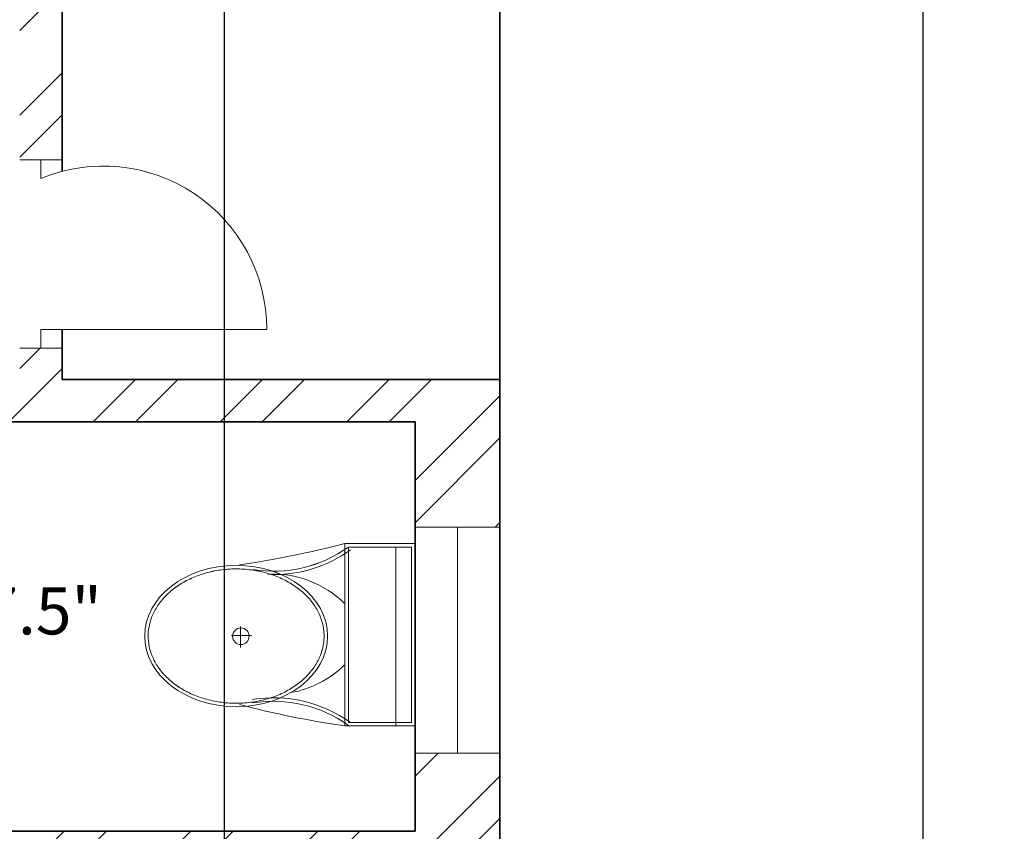
# Model space of a CAD drawing. Units: inches. Extents: x 2120 to 4013, y 1390 to 3019.
# Tile 25 of 59: x 2959 to 3063, y 1792 to 1878. Entities that reach past the tile are written whole.
import ezdxf

# ---------------------------------------------------------------- set-up
doc = ezdxf.new("R2010")
doc.units = ezdxf.units.IN
for name, color, linetype, lineweight in [('A-ANNO-DIMS', 2, 'Continuous', 18), ('A-AREA-IDEN', 7, 'Continuous', 18), ('A-DOOR', 3, 'Continuous', 18), ('A-FLOR-FIXT', 9, 'Continuous', 18), ('A-GLAZ', 4, 'Continuous', 18), ('A-WALL', 7, 'Continuous', 35), ('A-WALL-PATT', 252, 'Continuous', 13)]:
    doc.layers.add(name, color=color, linetype=linetype, lineweight=lineweight)
doc.styles.get("Standard").update_dxf_attribs({"font": 'arial.ttf'})
doc.dimstyles.get("Standard").update_dxf_attribs({"dimtxt": 0.18, "dimasz": 0.18, "dimexe": 0.18, "dimexo": 0.0625, "dimgap": 0.09, "dimtad": 0, "dimtih": 1, "dimtoh": 1, "dimdec": 4, "dimzin": 0, "dimdsep": 46, "dimtxsty": 'Standard', "dimcen": 0.09, "dimadec": 0, "dimazin": 0, "dimtfac": 1, "dimtdec": 4, "dimtofl": 0, "dimtmove": 0, "dimatfit": 3, "dimfxl": 1, "dimtolj": 1, "dimtzin": 0, "dimarcsym": 0})

# ---------------------------------------------------------------- blocks, each defined once
blk = doc.blocks.new('A$C31115884')
for p, q in [((257.5, 466.4), (257.5, 523.2)), ((283.1, 497.7), (223.4, 497.7)), ((0, 200), (0, 0)), ((520, 200), (0, 200)), ((520, 0), (520, 200)), ((10, 190), (10, 10)), ((510, 190), (10, 190)), ((510, 10), (510, 190)), ((510, 54.5), (0, 54.5)), ((10, 10), (510, 10)), ((0, 0), (520, 0))]:
    blk.add_line(p, q)
blk.add_circle((255.6, 496.4), 23.6)
for centre, radius, start, end in [((2777.7, -204.6), 2807, 165.4549, 171.7133), ((3237, 905), 2807, 188.2867, 194.5451), ((-294.5, 403.3), 364.7, 324.2091, 9.3499), ((-294.5, 403.3), 374.7, 324.2091, 9.3499), ((805.8, 403.3), 364.7, 170.6501, 215.7909), ((139.5, 406.2), 293.5, 315.8436, 2.6563), ((805.8, 403.3), 374.7, 179.2036, 215.7909), ((383.6, 406.2), 293.5, 190.2774, 224.1564)]:
    blk.add_arc(centre, radius, start, end)
blk.add_ellipse((256.2, 509.9), major_axis=(0, -260.7), ratio=0.772727)
blk.add_open_spline([(256.2, 259.2), (263.1, 259.2), (270, 259.7), (287.8, 262.3), (298.7, 265.1), (319.9, 273.1), (330.2, 278.4), (350.1, 291.1), (359.7, 298.7), (377.7, 315.9), (386.2, 325.5), (401.7, 346.6), (408.8, 358.1), (421.3, 382.5), (426.8, 395.5), (435.9, 422.4), (439.5, 436.4), (444.8, 465.1), (446.5, 479.7), (447.9, 509.2), (447.6, 524), (445, 553.3), (442.7, 567.8), (436.3, 596), (432.1, 609.7), (421.9, 636), (416, 648.6), (402.5, 672.1), (395, 683), (378.6, 703), (369.8, 712.1), (351.1, 728), (341.3, 734.8), (320.9, 746.2), (310.4, 750.7), (288.9, 757.3), (278, 759.4), (256, 761), (245, 760.6), (223.1, 757.2), (212.3, 754.3), (191.1, 746.1), (180.8, 740.7), (160.9, 727.8), (151.4, 720.1), (133.5, 702.7), (125.1, 693), (109.6, 671.7), (102.6, 660.2), (90.2, 635.7), (84.9, 622.7), (76, 595.6), (72.4, 581.6), (67.2, 552.9), (65.6, 538.2), (64.4, 508.8), (64.8, 494), (67.5, 464.7), (69.9, 450.2), (76.6, 422), (80.8, 408.3), (91.1, 382.2), (97.2, 369.7), (110.8, 346.3), (118.4, 335.4), (134.8, 315.6), (143.7, 306.7), (162.4, 290.9), (172.3, 284.2), (192.8, 273), (203.3, 268.6), (224.8, 262.2), (235.8, 260.2), (249.9, 259.3), (253, 259.2), (256.2, 259.2)], degree=3, knots=[0, 0, 0, 0, 0.110105, 0.110105, 0.285049, 0.285049, 0.459994, 0.459994, 0.634938, 0.634938, 0.809882, 0.809882, 0.984827, 0.984827, 1.159771, 1.159771, 1.334715, 1.334715, 1.50966, 1.50966, 1.684604, 1.684604, 1.859549, 1.859549, 2.034493, 2.034493, 2.209437, 2.209437, 2.384382, 2.384382, 2.559326, 2.559326, 2.73427, 2.73427, 2.909215, 2.909215, 3.084159, 3.084159, 3.259103, 3.259103, 3.434048, 3.434048, 3.608992, 3.608992, 3.783936, 3.783936, 3.958881, 3.958881, 4.133825, 4.133825, 4.30877, 4.30877, 4.483714, 4.483714, 4.658658, 4.658658, 4.833603, 4.833603, 5.008547, 5.008547, 5.183491, 5.183491, 5.358436, 5.358436, 5.53338, 5.53338, 5.708324, 5.708324, 5.883269, 5.883269, 6.058213, 6.058213, 6.233158, 6.233158, 6.283185, 6.283185, 6.283185, 6.283185])
blk = doc.blocks.new('DOOR-SWING-24IN-112p55DEG')
for p, q in [((0, 20.02), (4.5, 20.02)), ((4.5, 20.02), (2.25, 20.02)), ((2.25, 20.02), (2.25, 18.02)), ((2.25, 0), (2.25, 2)), ((2.25, 2), (26.25, 2)), ((0, 0), (4.5, 0)), ((4.5, 0), (2.25, 0))]:
    blk.add_line(p, q)
blk.add_arc((8.9, 2), 17.35, 0, 112.5501)
blk = doc.blocks.new('WIN-PLAN-24IN-05')
for p, q in [((4.5, 24), (0, 24)), ((0, 24), (9, 24)), ((4.5, 0), (4.5, 24)), ((0, 0), (9, 0)), ((9, 0), (0, 0)), ((0, 0), (4.5, 0))]:
    blk.add_line(p, q)
blk = doc.blocks.new('*D212')
at = {"layer": 'A-ANNO-DIMS', "color": 0, "lineweight": -2, "transparency": 16777216}
for p, q in [((3009.8, 2352.53), (3054.91, 2352.53)), ((3054.73, 2352.35), (3054.73, 1947.71)), ((3054.73, 1542.71), (3054.73, 1947.35)), ((3009.8, 1542.53), (3054.91, 1542.53))]:
    blk.add_line(p, q, dxfattribs=at)
at = {"layer": 'A-ANNO-DIMS', "color": 0, "transparency": 16777216}
for points in [[(3054.7, 2352.35), (3054.76, 2352.35), (3054.73, 2352.53)], [(3054.7, 1542.71), (3054.76, 1542.71), (3054.73, 1542.53)]]:
    blk.add_solid(points, dxfattribs=at)
at = {"layer": 'Defpoints', "color": 0, "transparency": 16777216}
for p in [(3009.73, 2352.53), (3009.73, 1542.53), (3054.73, 1542.53)]:
    blk.add_point(p, dxfattribs=at)
at = {"layer": 'A-ANNO-DIMS', "color": 0, "transparency": 16777216, "insert": (3054.73, 1947.53), "char_height": 0.18, "attachment_point": 5}
blk.add_mtext('\\A1;810', dxfattribs=at)
blk = doc.blocks.new('*D217')
at = {"layer": 'A-ANNO-DIMS', "color": 0, "lineweight": -2, "transparency": 16777216}
for p, q in [((3071.67, 2352.53), (2980.31, 2352.53)), ((2980.49, 2352.35), (2980.49, 1947.71)), ((2980.49, 1542.71), (2980.49, 1947.35)), ((3305.67, 1542.53), (2980.31, 1542.53))]:
    blk.add_line(p, q, dxfattribs=at)
at = {"layer": 'A-ANNO-DIMS', "color": 0, "transparency": 16777216}
for points in [[(2980.46, 2352.35), (2980.52, 2352.35), (2980.49, 2352.53)], [(2980.46, 1542.71), (2980.52, 1542.71), (2980.49, 1542.53)]]:
    blk.add_solid(points, dxfattribs=at)
at = {"layer": 'Defpoints', "color": 0, "transparency": 16777216}
for p in [(2980.49, 2352.53), (3071.73, 2352.53), (3305.73, 1542.53)]:
    blk.add_point(p, dxfattribs=at)
at = {"layer": 'A-ANNO-DIMS', "color": 0, "transparency": 16777216, "insert": (2980.49, 1947.53), "char_height": 0.18, "attachment_point": 5}
blk.add_mtext('\\A1;810', dxfattribs=at)

msp = doc.modelspace()

# ---------------------------------------------------------------- hatches: boundary and pattern name
at = {"layer": 'A-WALL-PATT'}
h = msp.add_hatch(dxfattribs=at)
h.set_pattern_fill('ANSI32', color=256)
h.paths.add_polyline_path([(2271.7331, 2343.531), (2283.3788, 2343.531), (2283.3788, 2348.031), (2283.3788, 2352.5306), (2262.7331, 2352.5306), (2262.7331, 2182.638), (2267.2331, 2182.638), (2271.7331, 2182.638), (2271.7331, 2219.031), (2391.7331, 2219.031), (2391.7331, 2214.189), (2393.9831, 2214.189), (2396.2331, 2214.189), (2396.2331, 2219.031), (2420.2331, 2219.031), (2420.2331, 2225.7535), (2417.2197, 2225.7535), (2415.7331, 2225.7535), (2415.7331, 2223.5306), (2271.7331, 2223.5306)])
h.paths.add_polyline_path([(2380.0942, 2352.5306), (2343.3788, 2352.5306), (2343.3788, 2343.531), (2363.2331, 2343.531), (2363.2331, 2288.8489), (2365.4831, 2288.8489), (2367.7331, 2288.8489), (2367.7331, 2343.531), (2380.0942, 2343.531)], flags=17)
h.paths.add_polyline_path([(2432.4339, 2352.5306), (2404.0943, 2352.5306), (2404.0943, 2343.531), (2415.7331, 2343.531), (2415.7331, 2264.0306), (2367.7331, 2264.0306), (2367.7331, 2266.4872), (2363.2331, 2266.4872), (2363.2331, 2259.531), (2367.7331, 2259.531), (2415.7331, 2259.531), (2415.7331, 2255.0658), (2420.2331, 2255.0658), (2420.2331, 2259.531), (2424.5717, 2259.531), (2424.5717, 2261.781), (2424.5717, 2264.0306), (2420.2331, 2264.0306), (2420.2331, 2343.531), (2432.4339, 2343.531)])
h.paths.add_polyline_path([(2508.9115, 2352.5306), (2456.4339, 2352.5306), (2456.4339, 2343.531), (2468.2331, 2343.531), (2468.2331, 2264.0306), (2448.0487, 2264.0306), (2448.0487, 2259.531), (2468.2331, 2259.531), (2468.2331, 2255.5496), (2472.7331, 2255.5496), (2472.7331, 2343.531), (2508.9115, 2343.531)])
h.paths.add_polyline_path([(2637.7331, 2352.5306), (2544.9116, 2352.5306), (2544.9116, 2343.531), (2589.7331, 2343.531), (2633.2331, 2343.531), (2637.7331, 2343.531)])
h.paths.add_polyline_path([(2594.2331, 2343.5306), (2589.7331, 2343.5306), (2589.7331, 2259.5306), (2589.7331, 2252.4915), (2591.9831, 2252.4915), (2594.2331, 2252.4915)])
h.paths.add_polyline_path([(2637.7331, 2223.5306), (2594.2331, 2223.5306), (2594.2331, 2230.1988), (2591.9831, 2230.1988), (2589.7331, 2230.1988), (2589.7331, 2223.5306), (2472.7331, 2223.5306), (2468.2331, 2223.5306), (2468.2331, 2219.031), (2628.7331, 2219.031), (2628.7331, 2138.031), (2637.7331, 2138.031)])
h.paths.add_polyline_path([(3822.6535, 2458.4402), (3874.9468, 2458.4402), (3874.9468, 2476.9866), (3822.6535, 2476.9866)], flags=9)
h.paths.add_polyline_path([(3834.6921, 2781.8174), (3935.9206, 2781.8174), (3935.9206, 2800.3638), (3834.6921, 2800.3638)], flags=9)
h.paths.add_polyline_path([(3832.2843, 2837.9683), (3884.5776, 2837.9683), (3884.5776, 2856.5146), (3832.2843, 2856.5146)], flags=9)
h.paths.add_polyline_path([(3830.9388, 2861.4782), (3956.8958, 2861.4782), (3956.8958, 2880.0245), (3830.9388, 2880.0245)], flags=9)
h.paths.add_polyline_path([(3870.6966, 2352.5752), (3887.9272, 2352.5752), (3887.9272, 2377.3037), (3870.6966, 2377.3037)], flags=9)
h.paths.add_polyline_path([(3289.2701, 2413.161), (3435.2223, 2413.161), (3435.2223, 2450.2538), (3289.2701, 2450.2538)], flags=9)
h.paths.add_polyline_path([(2487.6944, 2414.3601), (2637.8335, 2414.3601), (2637.8335, 2451.4528), (2487.6944, 2451.4528)], flags=9)
h.paths.add_polyline_path([(2567.3724, 1457.9199), (2815.296, 1457.9199), (2815.296, 1495.0127), (2567.3724, 1495.0127)], flags=9)
h.paths.add_polyline_path([(2655.3825, 2093.2363), (2685.9555, 2093.2363), (2685.9555, 2111.8937), (2655.3825, 2111.8937)], flags=9)
h.paths.add_polyline_path([(2543.9218, 1550.6671), (2587.8406, 1550.6671), (2587.8406, 1569.3244), (2543.9218, 1569.3244)], flags=9)
h.paths.add_polyline_path([(2905.1384, 1543.8113), (2949.0572, 1543.8113), (2949.0572, 1562.4686), (2905.1384, 1562.4686)], flags=9)
h.paths.add_polyline_path([(2736.4118, 1702.4736), (2784.2153, 1702.4736), (2784.2153, 1721.1309), (2736.4118, 1721.1309)], flags=9)
h.paths.add_polyline_path([(2912.8666, 1710.4168), (2951.707, 1710.4168), (2951.707, 1729.0741), (2912.8666, 1729.0741)], flags=9)
h.paths.add_polyline_path([(2923.5785, 1763.5038), (2959.7279, 1763.5038), (2959.7279, 1782.1611), (2923.5785, 1782.1611)], flags=9)
h.paths.add_polyline_path([(2925.2114, 1809.6137), (2967.1861, 1809.6137), (2967.1861, 1828.271), (2925.2114, 1828.271)], flags=9)
h.paths.add_polyline_path([(2996.2711, 1878.9003), (2996.2711, 1913.109), (2977.6138, 1913.109), (2977.6138, 1878.9003)], flags=9)
h.paths.add_polyline_path([(2883.0859, 1895.7192), (2927.1855, 1895.7192), (2927.1855, 1914.3766), (2883.0859, 1914.3766)], flags=9)
h.paths.add_polyline_path([(2787.3924, 1810.8013), (2841.0213, 1810.8013), (2841.0213, 1829.4587), (2787.3924, 1829.4587)], flags=9)
h.paths.add_polyline_path([(2775.6399, 2101.7395), (2829.2689, 2101.7395), (2829.2689, 2120.3968), (2775.6399, 2120.3968)], flags=9)
h.paths.add_polyline_path([(2913.0263, 2075.817), (2951.8667, 2075.817), (2951.8667, 2094.4744), (2913.0263, 2094.4744)], flags=9)
h.paths.add_polyline_path([(2929.966, 2133.3669), (2966.1154, 2133.3669), (2966.1154, 2152.0243), (2929.966, 2152.0243)], flags=9)
h.paths.add_polyline_path([(2932.7502, 2182.6088), (2968.8996, 2182.6088), (2968.8996, 2201.2662), (2932.7502, 2201.2662)], flags=9)
h.paths.add_polyline_path([(2996.0681, 2266.3173), (2996.0681, 2300.5261), (2977.4108, 2300.5261), (2977.4108, 2266.3173)], flags=9)
h.paths.add_polyline_path([(2885.1039, 2279.2186), (2929.2035, 2279.2186), (2929.2035, 2297.8759), (2885.1039, 2297.8759)], flags=9)
h.paths.add_polyline_path([(2735.7042, 2218.3197), (2783.5078, 2218.3197), (2783.5078, 2236.9771), (2735.7042, 2236.9771)], flags=9)
h.paths.add_polyline_path([(2635.6049, 2044.0085), (2648.9678, 2044.0085), (2648.9678, 2054.312), (2635.6049, 2054.312)], flags=9)
h.paths.add_polyline_path([(2714.0148, 1923.0473), (2727.3777, 1923.0473), (2727.3777, 1933.3508), (2714.0148, 1933.3508)], flags=9)
h.paths.add_polyline_path([(2709.0345, 1988.1628), (2722.3974, 1988.1628), (2722.3974, 1998.4663), (2709.0345, 1998.4663)], flags=9)
h.paths.add_polyline_path([(2592.8935, 1962.1763), (2606.2564, 1962.1763), (2606.2564, 1972.4799), (2592.8935, 1972.4799)], flags=9)
h.paths.add_polyline_path([(2618.3996, 1985.9724), (2644.1942, 1985.9724), (2644.1942, 1996.2759), (2618.3996, 1996.2759)], flags=9)
h.paths.add_polyline_path([(2601.279, 1920.5869), (2614.6419, 1920.5869), (2614.6419, 1930.8904), (2601.279, 1930.8904)], flags=9)
h.paths.add_polyline_path([(2692.3278, 1932.7645), (2704.5311, 1932.7645), (2704.5311, 1943.0681), (2692.3278, 1943.0681)], flags=9)
h.paths.add_polyline_path([(2311.122, 1672.7318), (2355.0408, 1672.7318), (2355.0408, 1691.3892), (2311.122, 1691.3892)], flags=9)
h.paths.add_polyline_path([(2456.2551, 1632.3198), (2492.4796, 1632.3198), (2492.4796, 1650.9772), (2456.2551, 1650.9772)], flags=9)
h.paths.add_polyline_path([(2401.0766, 1631.4793), (2437.301, 1631.4793), (2437.301, 1650.1367), (2401.0766, 1650.1367)], flags=9)
h.paths.add_polyline_path([(2546.7054, 1700.9235), (2594.509, 1700.9235), (2594.509, 1719.5809), (2546.7054, 1719.5809)], flags=9)
h.paths.add_polyline_path([(2445.4866, 1766.9937), (2497.5261, 1766.9937), (2497.5261, 1785.651), (2445.4866, 1785.651)], flags=9)
h.paths.add_polyline_path([(2287.9992, 1739.7675), (2326.8396, 1739.7675), (2326.8396, 1758.4248), (2287.9992, 1758.4248)], flags=9)
h.paths.add_polyline_path([(2458.5279, 1924.7607), (2510.5675, 1924.7607), (2510.5675, 1943.4181), (2458.5279, 1943.4181)], flags=9)
h.paths.add_polyline_path([(2309.2811, 1902.7642), (2345.4305, 1902.7642), (2345.4305, 1921.4215), (2309.2811, 1921.4215)], flags=9)
h.paths.add_polyline_path([(2490.7554, 2018.9392), (2530.7896, 2018.9392), (2530.7896, 2037.5965), (2490.7554, 2037.5965)], flags=9)
h.paths.add_polyline_path([(2402.143, 2024.7393), (2438.5414, 2024.7393), (2438.5414, 2043.3966), (2402.143, 2043.3966)], flags=9)
h.paths.add_polyline_path([(2287.856, 1931.7926), (2326.6964, 1931.7926), (2326.6964, 1950.4499), (2287.856, 1950.4499)], flags=9)
h.paths.add_polyline_path([(2281.7979, 2193.5771), (2320.6383, 2193.5771), (2320.6383, 2212.2344), (2281.7979, 2212.2344)], flags=25)
h.paths.add_polyline_path([(2484.0754, 2093.892), (2536.115, 2093.892), (2536.115, 2112.5494), (2484.0754, 2112.5494)], flags=9)
h.paths.add_polyline_path([(2624.7948, 2281.8639), (2624.7948, 2311.4137), (2606.1375, 2311.4137), (2606.1375, 2281.8639)], flags=9)
h.paths.add_polyline_path([(2507.5036, 2290.3639), (2541.934, 2290.3639), (2541.934, 2309.0212), (2507.5036, 2309.0212)], flags=9)
h.paths.add_polyline_path([(2423.1076, 2285.2202), (2459.332, 2285.2202), (2459.332, 2303.8776), (2423.1076, 2303.8776)], flags=9)
h.paths.add_polyline_path([(2374.5467, 2289.6272), (2410.7711, 2289.6272), (2410.7711, 2308.2846), (2374.5467, 2308.2846)], flags=25)
h.paths.add_polyline_path([(2277.4907, 2227.5651), (2316.3311, 2227.5651), (2316.3311, 2246.2224), (2277.4907, 2246.2224)], flags=25)
h.paths.add_polyline_path([(2655.3825, 2093.2367), (2685.9555, 2093.2367), (2685.9555, 2111.894), (2655.3825, 2111.894)], flags=9)
h.paths.add_polyline_path([(2543.9217, 1550.6674), (2587.8406, 1550.6674), (2587.8406, 1569.3247), (2543.9217, 1569.3247)], flags=9)
h.paths.add_polyline_path([(2905.1384, 1543.8116), (2949.0572, 1543.8116), (2949.0572, 1562.4689), (2905.1384, 1562.4689)], flags=9)
h.paths.add_polyline_path([(2736.4118, 1702.4739), (2784.2153, 1702.4739), (2784.2153, 1721.1312), (2736.4118, 1721.1312)], flags=9)
h.paths.add_polyline_path([(2912.8666, 1710.4171), (2951.707, 1710.4171), (2951.707, 1729.0744), (2912.8666, 1729.0744)], flags=9)
h.paths.add_polyline_path([(2923.5785, 1763.5041), (2959.7279, 1763.5041), (2959.7279, 1782.1614), (2923.5785, 1782.1614)], flags=9)
h.paths.add_polyline_path([(2925.2114, 1809.614), (2967.1861, 1809.614), (2967.1861, 1828.2713), (2925.2114, 1828.2713)], flags=9)
h.paths.add_polyline_path([(2996.2711, 1878.9006), (2996.2711, 1913.1094), (2977.6137, 1913.1094), (2977.6137, 1878.9006)], flags=9)
h.paths.add_polyline_path([(2883.0859, 1895.7195), (2927.1855, 1895.7195), (2927.1855, 1914.3769), (2883.0859, 1914.3769)], flags=9)
h.paths.add_polyline_path([(2787.3924, 1810.8016), (2841.0213, 1810.8016), (2841.0213, 1829.459), (2787.3924, 1829.459)], flags=9)
h.paths.add_polyline_path([(2775.6399, 2101.7398), (2829.2688, 2101.7398), (2829.2688, 2120.3971), (2775.6399, 2120.3971)], flags=9)
h.paths.add_polyline_path([(2913.0263, 2075.8173), (2951.8667, 2075.8173), (2951.8667, 2094.4747), (2913.0263, 2094.4747)], flags=9)
h.paths.add_polyline_path([(2929.966, 2133.3672), (2966.1154, 2133.3672), (2966.1154, 2152.0246), (2929.966, 2152.0246)], flags=9)
h.paths.add_polyline_path([(2932.7502, 2182.6091), (2968.8996, 2182.6091), (2968.8996, 2201.2665), (2932.7502, 2201.2665)], flags=9)
h.paths.add_polyline_path([(2996.0681, 2266.3176), (2996.0681, 2300.5264), (2977.4108, 2300.5264), (2977.4108, 2266.3176)], flags=9)
h.paths.add_polyline_path([(2885.1039, 2279.2189), (2929.2035, 2279.2189), (2929.2035, 2297.8762), (2885.1039, 2297.8762)], flags=9)
h.paths.add_polyline_path([(2735.7042, 2218.32), (2783.5078, 2218.32), (2783.5078, 2236.9774), (2735.7042, 2236.9774)], flags=9)
h.paths.add_polyline_path([(2635.6048, 2044.0088), (2648.9677, 2044.0088), (2648.9677, 2054.3123), (2635.6048, 2054.3123)], flags=9)
h.paths.add_polyline_path([(2714.0148, 1923.0476), (2727.3777, 1923.0476), (2727.3777, 1933.3511), (2714.0148, 1933.3511)], flags=9)
h.paths.add_polyline_path([(2709.0345, 1988.1631), (2722.3974, 1988.1631), (2722.3974, 1998.4666), (2709.0345, 1998.4666)], flags=9)
h.paths.add_polyline_path([(2592.8935, 1962.1766), (2606.2564, 1962.1766), (2606.2564, 1972.4802), (2592.8935, 1972.4802)], flags=9)
h.paths.add_polyline_path([(2618.3995, 1985.9727), (2644.1942, 1985.9727), (2644.1942, 1996.2762), (2618.3995, 1996.2762)], flags=9)
h.paths.add_polyline_path([(2601.279, 1920.5872), (2614.6419, 1920.5872), (2614.6419, 1930.8908), (2601.279, 1930.8908)], flags=9)
h.paths.add_polyline_path([(2692.3278, 1932.7648), (2704.5311, 1932.7648), (2704.5311, 1943.0684), (2692.3278, 1943.0684)], flags=9)
h.paths.add_polyline_path([(2311.122, 1672.7321), (2355.0408, 1672.7321), (2355.0408, 1691.3895), (2311.122, 1691.3895)], flags=9)
h.paths.add_polyline_path([(2456.2551, 1632.3201), (2492.4795, 1632.3201), (2492.4795, 1650.9775), (2456.2551, 1650.9775)], flags=9)
h.paths.add_polyline_path([(2401.0766, 1631.4796), (2437.301, 1631.4796), (2437.301, 1650.137), (2401.0766, 1650.137)], flags=9)
h.paths.add_polyline_path([(2546.7054, 1700.9238), (2594.509, 1700.9238), (2594.509, 1719.5812), (2546.7054, 1719.5812)], flags=9)
h.paths.add_polyline_path([(2445.4866, 1766.994), (2497.5261, 1766.994), (2497.5261, 1785.6513), (2445.4866, 1785.6513)], flags=9)
h.paths.add_polyline_path([(2287.9992, 1739.7678), (2326.8396, 1739.7678), (2326.8396, 1758.4251), (2287.9992, 1758.4251)], flags=9)
h.paths.add_polyline_path([(2458.5279, 1924.7611), (2510.5675, 1924.7611), (2510.5675, 1943.4184), (2458.5279, 1943.4184)], flags=9)
h.paths.add_polyline_path([(2309.2811, 1902.7645), (2345.4305, 1902.7645), (2345.4305, 1921.4218), (2309.2811, 1921.4218)], flags=9)
h.paths.add_polyline_path([(2490.7554, 2018.9395), (2530.7895, 2018.9395), (2530.7895, 2037.5968), (2490.7554, 2037.5968)], flags=9)
h.paths.add_polyline_path([(2402.143, 2024.7396), (2438.5413, 2024.7396), (2438.5413, 2043.3969), (2402.143, 2043.3969)], flags=9)
h.paths.add_polyline_path([(2287.856, 1931.7929), (2326.6964, 1931.7929), (2326.6964, 1950.4502), (2287.856, 1950.4502)], flags=9)
h.paths.add_polyline_path([(2281.7979, 2193.5774), (2320.6383, 2193.5774), (2320.6383, 2212.2347), (2281.7979, 2212.2347)], flags=25)
h.paths.add_polyline_path([(2484.0754, 2093.8924), (2536.115, 2093.8924), (2536.115, 2112.5497), (2484.0754, 2112.5497)], flags=9)
h.paths.add_polyline_path([(2624.7948, 2281.8642), (2624.7948, 2311.414), (2606.1374, 2311.414), (2606.1374, 2281.8642)], flags=9)
h.paths.add_polyline_path([(2507.5035, 2290.3642), (2541.934, 2290.3642), (2541.934, 2309.0215), (2507.5035, 2309.0215)], flags=9)
h.paths.add_polyline_path([(2423.1075, 2285.2205), (2459.332, 2285.2205), (2459.332, 2303.8779), (2423.1075, 2303.8779)], flags=9)
h.paths.add_polyline_path([(2374.5467, 2289.6275), (2410.7711, 2289.6275), (2410.7711, 2308.2849), (2374.5467, 2308.2849)], flags=25)
h.paths.add_polyline_path([(2277.4907, 2227.5654), (2316.3311, 2227.5654), (2316.3311, 2246.2227), (2277.4907, 2246.2227)], flags=25)
h = msp.add_hatch(dxfattribs=at)
h.set_pattern_fill('ANSI32', color=256)
h.paths.add_polyline_path([(2271.7331, 1980.389), (2262.7331, 1980.389), (2262.7331, 1912.8434), (2267.2331, 1912.8434), (2271.7331, 1912.8434), (2271.7331, 1922.531), (2351.2331, 1922.531), (2351.2331, 1901.4728), (2355.7331, 1901.4728), (2355.7331, 1922.531), (2357.9815, 1922.531), (2357.9815, 1926.5306), (2271.7331, 1926.5306)])
h.paths.add_polyline_path([(2589.2331, 1949.1622), (2584.7331, 1949.1622), (2580.2331, 1949.1622), (2580.2331, 1874.5306), (2355.7331, 1874.5306), (2355.7331, 1880.1922), (2351.2331, 1880.1922), (2351.2331, 1874.5306), (2271.7331, 1874.5306), (2271.7331, 1888.8431), (2262.7331, 1888.8431), (2262.7331, 1842.2909), (2267.2331, 1842.2909), (2271.7331, 1842.2909), (2271.7331, 1865.531), (2415.7331, 1865.531), (2415.7331, 1779.7286), (2420.2331, 1779.7286), (2420.2331, 1865.531), (2589.2331, 1865.531)])
h.paths.add_polyline_path([(2271.7331, 1782.2906), (2262.7331, 1782.2906), (2262.7331, 1711.4639), (2267.2331, 1711.4639), (2271.7331, 1711.4639), (2271.7331, 1738.031), (2420.2331, 1738.031), (2420.2331, 1742.531), (2420.2331, 1747.3376), (2417.9831, 1747.3376), (2415.7331, 1747.3376), (2415.7331, 1742.5306), (2271.7331, 1742.5306)])
h.paths.add_polyline_path([(2271.7331, 1627.031), (2362.3957, 1627.031), (2362.3957, 1629.281), (2362.3957, 1631.5306), (2271.7331, 1631.5306), (2271.7331, 1675.4636), (2262.7331, 1675.4636), (2262.7331, 1581.531), (2405.3032, 1581.531), (2405.3032, 1586.031), (2405.3032, 1590.5306), (2396.2331, 1590.5306), (2396.2331, 1691.4513), (2418.7206, 1691.4513), (2418.7206, 1695.951), (2396.2331, 1695.951), (2391.7331, 1695.951), (2391.7331, 1631.5306), (2386.7425, 1631.5306), (2386.7425, 1629.2806), (2386.7425, 1627.031), (2391.7331, 1627.031), (2391.7331, 1586.1709), (2271.7331, 1586.1709)])
h.paths.add_polyline_path([(2459.6703, 1590.5306), (2429.3032, 1590.5306), (2429.3032, 1581.531), (2459.6703, 1581.531), (2459.6703, 1586.031)])
h.paths.add_polyline_path([(2501.2331, 1590.531), (2501.2331, 1665.0195), (2498.9831, 1665.0195), (2496.7331, 1665.0195), (2496.7331, 1590.5306), (2483.8201, 1590.5306), (2483.8201, 1590.1579), (2483.6704, 1590.1579), (2483.6704, 1581.531), (2505.0196, 1581.531), (2505.0196, 1583.781), (2505.0196, 1586.0306), (2501.2331, 1586.0306)])
h.paths.add_polyline_path([(2544.1361, 1583.781), (2544.1361, 1586.0306), (2527.1368, 1586.0306), (2527.1368, 1583.7806), (2527.1368, 1581.531), (2544.1361, 1581.531)])
h.paths.add_polyline_path([(3822.6535, 2458.4402), (3874.9468, 2458.4402), (3874.9468, 2476.9866), (3822.6535, 2476.9866)], flags=9)
h.paths.add_polyline_path([(3834.6921, 2781.8174), (3935.9206, 2781.8174), (3935.9206, 2800.3638), (3834.6921, 2800.3638)], flags=9)
h.paths.add_polyline_path([(3832.2843, 2837.9683), (3884.5776, 2837.9683), (3884.5776, 2856.5146), (3832.2843, 2856.5146)], flags=9)
h.paths.add_polyline_path([(3830.9388, 2861.4782), (3956.8958, 2861.4782), (3956.8958, 2880.0245), (3830.9388, 2880.0245)], flags=9)
h.paths.add_polyline_path([(3870.6966, 2352.5752), (3887.9272, 2352.5752), (3887.9272, 2377.3037), (3870.6966, 2377.3037)], flags=9)
h.paths.add_polyline_path([(3289.2701, 2413.161), (3435.2223, 2413.161), (3435.2223, 2450.2538), (3289.2701, 2450.2538)], flags=9)
h.paths.add_polyline_path([(2487.6944, 2414.3601), (2637.8335, 2414.3601), (2637.8335, 2451.4528), (2487.6944, 2451.4528)], flags=9)
h.paths.add_polyline_path([(2567.3724, 1457.9199), (2815.296, 1457.9199), (2815.296, 1495.0127), (2567.3724, 1495.0127)], flags=9)
h.paths.add_polyline_path([(2655.3825, 2093.2363), (2685.9555, 2093.2363), (2685.9555, 2111.8937), (2655.3825, 2111.8937)], flags=9)
h.paths.add_polyline_path([(2543.9218, 1550.6671), (2587.8406, 1550.6671), (2587.8406, 1569.3244), (2543.9218, 1569.3244)], flags=9)
h.paths.add_polyline_path([(2905.1384, 1543.8113), (2949.0572, 1543.8113), (2949.0572, 1562.4686), (2905.1384, 1562.4686)], flags=9)
h.paths.add_polyline_path([(2736.4118, 1702.4736), (2784.2153, 1702.4736), (2784.2153, 1721.1309), (2736.4118, 1721.1309)], flags=9)
h.paths.add_polyline_path([(2912.8666, 1710.4168), (2951.707, 1710.4168), (2951.707, 1729.0741), (2912.8666, 1729.0741)], flags=9)
h.paths.add_polyline_path([(2923.5785, 1763.5038), (2959.7279, 1763.5038), (2959.7279, 1782.1611), (2923.5785, 1782.1611)], flags=9)
h.paths.add_polyline_path([(2925.2114, 1809.6137), (2967.1861, 1809.6137), (2967.1861, 1828.271), (2925.2114, 1828.271)], flags=9)
h.paths.add_polyline_path([(2996.2711, 1878.9003), (2996.2711, 1913.109), (2977.6138, 1913.109), (2977.6138, 1878.9003)], flags=9)
h.paths.add_polyline_path([(2883.0859, 1895.7192), (2927.1855, 1895.7192), (2927.1855, 1914.3766), (2883.0859, 1914.3766)], flags=9)
h.paths.add_polyline_path([(2787.3924, 1810.8013), (2841.0213, 1810.8013), (2841.0213, 1829.4587), (2787.3924, 1829.4587)], flags=9)
h.paths.add_polyline_path([(2775.6399, 2101.7395), (2829.2689, 2101.7395), (2829.2689, 2120.3968), (2775.6399, 2120.3968)], flags=9)
h.paths.add_polyline_path([(2913.0263, 2075.817), (2951.8667, 2075.817), (2951.8667, 2094.4744), (2913.0263, 2094.4744)], flags=9)
h.paths.add_polyline_path([(2929.966, 2133.3669), (2966.1154, 2133.3669), (2966.1154, 2152.0243), (2929.966, 2152.0243)], flags=9)
h.paths.add_polyline_path([(2932.7502, 2182.6088), (2968.8996, 2182.6088), (2968.8996, 2201.2662), (2932.7502, 2201.2662)], flags=9)
h.paths.add_polyline_path([(2996.0681, 2266.3173), (2996.0681, 2300.5261), (2977.4108, 2300.5261), (2977.4108, 2266.3173)], flags=9)
h.paths.add_polyline_path([(2885.1039, 2279.2186), (2929.2035, 2279.2186), (2929.2035, 2297.8759), (2885.1039, 2297.8759)], flags=9)
h.paths.add_polyline_path([(2735.7042, 2218.3197), (2783.5078, 2218.3197), (2783.5078, 2236.9771), (2735.7042, 2236.9771)], flags=9)
h.paths.add_polyline_path([(2635.6049, 2044.0085), (2648.9678, 2044.0085), (2648.9678, 2054.312), (2635.6049, 2054.312)], flags=9)
h.paths.add_polyline_path([(2714.0148, 1923.0473), (2727.3777, 1923.0473), (2727.3777, 1933.3508), (2714.0148, 1933.3508)], flags=9)
h.paths.add_polyline_path([(2709.0345, 1988.1628), (2722.3974, 1988.1628), (2722.3974, 1998.4663), (2709.0345, 1998.4663)], flags=9)
h.paths.add_polyline_path([(2592.8935, 1962.1763), (2606.2564, 1962.1763), (2606.2564, 1972.4799), (2592.8935, 1972.4799)], flags=9)
h.paths.add_polyline_path([(2618.3996, 1985.9724), (2644.1942, 1985.9724), (2644.1942, 1996.2759), (2618.3996, 1996.2759)], flags=9)
h.paths.add_polyline_path([(2601.279, 1920.5869), (2614.6419, 1920.5869), (2614.6419, 1930.8904), (2601.279, 1930.8904)], flags=9)
h.paths.add_polyline_path([(2692.3278, 1932.7645), (2704.5311, 1932.7645), (2704.5311, 1943.0681), (2692.3278, 1943.0681)], flags=9)
h.paths.add_polyline_path([(2311.122, 1672.7318), (2355.0408, 1672.7318), (2355.0408, 1691.3892), (2311.122, 1691.3892)], flags=25)
h.paths.add_polyline_path([(2456.2551, 1632.3198), (2492.4796, 1632.3198), (2492.4796, 1650.9772), (2456.2551, 1650.9772)], flags=9)
h.paths.add_polyline_path([(2401.0766, 1631.4793), (2437.301, 1631.4793), (2437.301, 1650.1367), (2401.0766, 1650.1367)], flags=9)
h.paths.add_polyline_path([(2546.7054, 1700.9235), (2594.509, 1700.9235), (2594.509, 1719.5809), (2546.7054, 1719.5809)], flags=9)
h.paths.add_polyline_path([(2445.4866, 1766.9937), (2497.5261, 1766.9937), (2497.5261, 1785.651), (2445.4866, 1785.651)], flags=9)
h.paths.add_polyline_path([(2287.9992, 1739.7675), (2326.8396, 1739.7675), (2326.8396, 1758.4248), (2287.9992, 1758.4248)], flags=24)
h.paths.add_polyline_path([(2458.5279, 1924.7607), (2510.5675, 1924.7607), (2510.5675, 1943.4181), (2458.5279, 1943.4181)], flags=25)
h.paths.add_polyline_path([(2309.2811, 1902.7642), (2345.4305, 1902.7642), (2345.4305, 1921.4215), (2309.2811, 1921.4215)], flags=25)
h.paths.add_polyline_path([(2490.7554, 2018.9392), (2530.7896, 2018.9392), (2530.7896, 2037.5965), (2490.7554, 2037.5965)], flags=9)
h.paths.add_polyline_path([(2402.143, 2024.7393), (2438.5414, 2024.7393), (2438.5414, 2043.3966), (2402.143, 2043.3966)], flags=9)
h.paths.add_polyline_path([(2287.856, 1931.7926), (2326.6964, 1931.7926), (2326.6964, 1950.4499), (2287.856, 1950.4499)], flags=25)
h.paths.add_polyline_path([(2281.7979, 2193.5771), (2320.6383, 2193.5771), (2320.6383, 2212.2344), (2281.7979, 2212.2344)], flags=9)
h.paths.add_polyline_path([(2484.0754, 2093.892), (2536.115, 2093.892), (2536.115, 2112.5494), (2484.0754, 2112.5494)], flags=9)
h.paths.add_polyline_path([(2624.7948, 2281.8639), (2624.7948, 2311.4137), (2606.1375, 2311.4137), (2606.1375, 2281.8639)], flags=9)
h.paths.add_polyline_path([(2507.5036, 2290.3639), (2541.934, 2290.3639), (2541.934, 2309.0212), (2507.5036, 2309.0212)], flags=9)
h.paths.add_polyline_path([(2423.1076, 2285.2202), (2459.332, 2285.2202), (2459.332, 2303.8776), (2423.1076, 2303.8776)], flags=9)
h.paths.add_polyline_path([(2374.5467, 2289.6272), (2410.7711, 2289.6272), (2410.7711, 2308.2846), (2374.5467, 2308.2846)], flags=9)
h.paths.add_polyline_path([(2277.4907, 2227.5651), (2316.3311, 2227.5651), (2316.3311, 2246.2224), (2277.4907, 2246.2224)], flags=9)
h.paths.add_polyline_path([(2655.3825, 2093.2367), (2685.9555, 2093.2367), (2685.9555, 2111.894), (2655.3825, 2111.894)], flags=9)
h.paths.add_polyline_path([(2543.9217, 1550.6674), (2587.8406, 1550.6674), (2587.8406, 1569.3247), (2543.9217, 1569.3247)], flags=9)
h.paths.add_polyline_path([(2905.1384, 1543.8116), (2949.0572, 1543.8116), (2949.0572, 1562.4689), (2905.1384, 1562.4689)], flags=9)
h.paths.add_polyline_path([(2736.4118, 1702.4739), (2784.2153, 1702.4739), (2784.2153, 1721.1312), (2736.4118, 1721.1312)], flags=9)
h.paths.add_polyline_path([(2912.8666, 1710.4171), (2951.707, 1710.4171), (2951.707, 1729.0744), (2912.8666, 1729.0744)], flags=9)
h.paths.add_polyline_path([(2923.5785, 1763.5041), (2959.7279, 1763.5041), (2959.7279, 1782.1614), (2923.5785, 1782.1614)], flags=9)
h.paths.add_polyline_path([(2925.2114, 1809.614), (2967.1861, 1809.614), (2967.1861, 1828.2713), (2925.2114, 1828.2713)], flags=9)
h.paths.add_polyline_path([(2996.2711, 1878.9006), (2996.2711, 1913.1094), (2977.6137, 1913.1094), (2977.6137, 1878.9006)], flags=9)
h.paths.add_polyline_path([(2883.0859, 1895.7195), (2927.1855, 1895.7195), (2927.1855, 1914.3769), (2883.0859, 1914.3769)], flags=9)
h.paths.add_polyline_path([(2787.3924, 1810.8016), (2841.0213, 1810.8016), (2841.0213, 1829.459), (2787.3924, 1829.459)], flags=9)
h.paths.add_polyline_path([(2775.6399, 2101.7398), (2829.2688, 2101.7398), (2829.2688, 2120.3971), (2775.6399, 2120.3971)], flags=9)
h.paths.add_polyline_path([(2913.0263, 2075.8173), (2951.8667, 2075.8173), (2951.8667, 2094.4747), (2913.0263, 2094.4747)], flags=9)
h.paths.add_polyline_path([(2929.966, 2133.3672), (2966.1154, 2133.3672), (2966.1154, 2152.0246), (2929.966, 2152.0246)], flags=9)
h.paths.add_polyline_path([(2932.7502, 2182.6091), (2968.8996, 2182.6091), (2968.8996, 2201.2665), (2932.7502, 2201.2665)], flags=9)
h.paths.add_polyline_path([(2996.0681, 2266.3176), (2996.0681, 2300.5264), (2977.4108, 2300.5264), (2977.4108, 2266.3176)], flags=9)
h.paths.add_polyline_path([(2885.1039, 2279.2189), (2929.2035, 2279.2189), (2929.2035, 2297.8762), (2885.1039, 2297.8762)], flags=9)
h.paths.add_polyline_path([(2735.7042, 2218.32), (2783.5078, 2218.32), (2783.5078, 2236.9774), (2735.7042, 2236.9774)], flags=9)
h.paths.add_polyline_path([(2635.6048, 2044.0088), (2648.9677, 2044.0088), (2648.9677, 2054.3123), (2635.6048, 2054.3123)], flags=9)
h.paths.add_polyline_path([(2714.0148, 1923.0476), (2727.3777, 1923.0476), (2727.3777, 1933.3511), (2714.0148, 1933.3511)], flags=9)
h.paths.add_polyline_path([(2709.0345, 1988.1631), (2722.3974, 1988.1631), (2722.3974, 1998.4666), (2709.0345, 1998.4666)], flags=9)
h.paths.add_polyline_path([(2592.8935, 1962.1766), (2606.2564, 1962.1766), (2606.2564, 1972.4802), (2592.8935, 1972.4802)], flags=9)
h.paths.add_polyline_path([(2618.3995, 1985.9727), (2644.1942, 1985.9727), (2644.1942, 1996.2762), (2618.3995, 1996.2762)], flags=9)
h.paths.add_polyline_path([(2601.279, 1920.5872), (2614.6419, 1920.5872), (2614.6419, 1930.8908), (2601.279, 1930.8908)], flags=9)
h.paths.add_polyline_path([(2692.3278, 1932.7648), (2704.5311, 1932.7648), (2704.5311, 1943.0684), (2692.3278, 1943.0684)], flags=9)
h.paths.add_polyline_path([(2311.122, 1672.7321), (2355.0408, 1672.7321), (2355.0408, 1691.3895), (2311.122, 1691.3895)], flags=25)
h.paths.add_polyline_path([(2456.2551, 1632.3201), (2492.4795, 1632.3201), (2492.4795, 1650.9775), (2456.2551, 1650.9775)], flags=9)
h.paths.add_polyline_path([(2401.0766, 1631.4796), (2437.301, 1631.4796), (2437.301, 1650.137), (2401.0766, 1650.137)], flags=9)
h.paths.add_polyline_path([(2546.7054, 1700.9238), (2594.509, 1700.9238), (2594.509, 1719.5812), (2546.7054, 1719.5812)], flags=9)
h.paths.add_polyline_path([(2445.4866, 1766.994), (2497.5261, 1766.994), (2497.5261, 1785.6513), (2445.4866, 1785.6513)], flags=9)
h.paths.add_polyline_path([(2287.9992, 1739.7678), (2326.8396, 1739.7678), (2326.8396, 1758.4251), (2287.9992, 1758.4251)], flags=24)
h.paths.add_polyline_path([(2458.5279, 1924.7611), (2510.5675, 1924.7611), (2510.5675, 1943.4184), (2458.5279, 1943.4184)], flags=25)
h.paths.add_polyline_path([(2309.2811, 1902.7645), (2345.4305, 1902.7645), (2345.4305, 1921.4218), (2309.2811, 1921.4218)], flags=25)
h.paths.add_polyline_path([(2490.7554, 2018.9395), (2530.7895, 2018.9395), (2530.7895, 2037.5968), (2490.7554, 2037.5968)], flags=9)
h.paths.add_polyline_path([(2402.143, 2024.7396), (2438.5413, 2024.7396), (2438.5413, 2043.3969), (2402.143, 2043.3969)], flags=9)
h.paths.add_polyline_path([(2287.856, 1931.7929), (2326.6964, 1931.7929), (2326.6964, 1950.4502), (2287.856, 1950.4502)], flags=25)
h.paths.add_polyline_path([(2281.7979, 2193.5774), (2320.6383, 2193.5774), (2320.6383, 2212.2347), (2281.7979, 2212.2347)], flags=9)
h.paths.add_polyline_path([(2484.0754, 2093.8924), (2536.115, 2093.8924), (2536.115, 2112.5497), (2484.0754, 2112.5497)], flags=9)
h.paths.add_polyline_path([(2624.7948, 2281.8642), (2624.7948, 2311.414), (2606.1374, 2311.414), (2606.1374, 2281.8642)], flags=9)
h.paths.add_polyline_path([(2507.5035, 2290.3642), (2541.934, 2290.3642), (2541.934, 2309.0215), (2507.5035, 2309.0215)], flags=9)
h.paths.add_polyline_path([(2423.1075, 2285.2205), (2459.332, 2285.2205), (2459.332, 2303.8779), (2423.1075, 2303.8779)], flags=9)
h.paths.add_polyline_path([(2374.5467, 2289.6275), (2410.7711, 2289.6275), (2410.7711, 2308.2849), (2374.5467, 2308.2849)], flags=9)
h.paths.add_polyline_path([(2277.4907, 2227.5654), (2316.3311, 2227.5654), (2316.3311, 2246.2227), (2277.4907, 2246.2227)], flags=9)
h = msp.add_hatch(dxfattribs=at)
h.set_pattern_fill('ANSI32', color=256)
h.paths.add_polyline_path([(2271.7331, 2122.6377), (2262.7331, 2122.6377), (2262.7331, 2040.3893), (2267.2331, 2040.3893), (2271.7331, 2040.3893), (2271.7331, 2044.8856), (2271.7331, 2070.531), (2391.7331, 2070.531), (2391.7331, 1926.5306), (2388.3993, 1926.5306), (2388.3993, 1922.531), (2395.7331, 1922.531), (2395.7331, 1992.531), (2400.4511, 1992.531), (2400.4511, 1997.0306), (2395.7331, 1997.0306), (2395.7331, 2070.531), (2443.7331, 2070.531), (2443.7331, 2046.1368), (2448.2331, 2046.1368), (2448.2331, 2070.531), (2580.2331, 2070.531), (2580.2331, 1997.0306), (2492.9076, 1997.0306), (2492.9076, 1992.531), (2580.2331, 1992.531), (2580.2331, 1983.9368), (2589.2331, 1983.9368), (2589.2331, 2070.531), (2589.2331, 2075.0306), (2396.2331, 2075.0306), (2396.2331, 2184.3565), (2393.9831, 2184.3565), (2391.7331, 2184.3565), (2391.7331, 2075.0306), (2271.7331, 2075.0306)])
h.paths.add_polyline_path([(2724.7331, 2138.0306), (2628.7331, 2138.0306), (2628.7331, 2070.5306), (2628.7331, 2067.0987), (2633.2331, 2067.0987), (2637.7331, 2067.0987), (2637.7331, 2070.531), (2657.3413, 2070.531), (2657.3413, 2079.5306), (2637.7331, 2079.5306), (2637.7331, 2129.031), (2715.7331, 2129.031), (2715.7331, 2079.5306), (2698.0378, 2079.5306), (2698.0378, 2070.531), (2715.7331, 2070.531), (2715.7331, 2012.1531), (2720.2331, 2012.1531), (2724.7331, 2012.1531)])
h.paths.add_polyline_path([(2724.7331, 2213.031), (2831.3209, 2213.031), (2831.3209, 2215.281), (2831.3209, 2217.5306), (2724.7331, 2217.5306), (2724.7331, 2343.531), (2751.8755, 2343.531), (2751.8755, 2352.5306), (2715.7331, 2352.5306), (2715.7331, 2138.031), (2724.7331, 2138.031)])
h.paths.add_polyline_path([(2902.53, 2352.5306), (2811.8755, 2352.5306), (2811.8755, 2343.531), (2867.2331, 2343.531), (2867.2331, 2217.5306), (2863.6364, 2217.5306), (2863.6364, 2213.031), (2871.7331, 2213.031), (2871.7331, 2217.531), (2871.7331, 2343.531), (2902.53, 2343.531)])
h.paths.add_polyline_path([(3009.7331, 2352.5306), (2938.53, 2352.5306), (2938.53, 2343.531), (2966.2331, 2343.531), (2966.2331, 2242.3281), (2968.4831, 2242.3281), (2970.7331, 2242.3281), (2970.7331, 2343.531), (3009.7331, 2343.531)])
h.paths.add_polyline_path([(3009.7331, 2217.5306), (2970.7331, 2217.5306), (2970.7331, 2220.5422), (2968.4831, 2220.5422), (2966.2331, 2220.5422), (2966.2331, 2217.5306), (2911.7752, 2217.5306), (2907.7331, 2217.5306), (2907.7331, 2213.0306), (2907.7331, 2194.9663), (2912.2331, 2194.9663), (2912.2331, 2213.031), (2970.7331, 2213.031), (3000.7331, 2213.031), (3000.7331, 2205.523), (3009.7331, 2205.523)])
h.paths.add_polyline_path([(3009.7331, 2181.5227), (3000.7331, 2181.5227), (3000.7331, 2165.0306), (2912.2331, 2165.0306), (2912.2331, 2170.8202), (2907.7331, 2170.8202), (2907.7331, 2165.0306), (2899.5169, 2165.0306), (2899.5169, 2162.7806), (2899.5169, 2160.531), (2907.7331, 2160.531), (2907.7331, 2137.3432), (2912.2331, 2137.3432), (2912.2331, 2160.531), (3000.7331, 2160.531), (3000.7331, 2150.4993), (3009.7331, 2150.4993)])
h.paths.add_polyline_path([(3009.7331, 2126.499), (3005.2331, 2126.499), (3000.7331, 2126.499), (3000.7331, 2112.5306), (2912.2331, 2112.5306), (2912.2331, 2115.6036), (2907.7331, 2115.6036), (2907.7331, 2108.031), (3000.7331, 2108.031), (3000.7331, 2084.7256), (3009.7331, 2084.7256)], flags=17)
h.paths.add_polyline_path([(3009.7331, 1971.531), (3009.7331, 2024.7253), (3000.7331, 2024.7253), (3000.7331, 2006.4153), (3000.7331, 1971.5306), (2864.2331, 1971.5306), (2864.2331, 2160.531), (2868.0522, 2160.531), (2868.0522, 2165.0306), (2859.7331, 2165.0306), (2859.7331, 1971.5306), (2724.7331, 1971.5306), (2724.7331, 1977.7012), (2715.7331, 1977.7012), (2715.7331, 1962.5306), (2715.7331, 1950.9035), (2720.2331, 1950.9035), (2724.7331, 1950.9035), (2724.7331, 1962.531), (2855.2331, 1962.531), (2859.7331, 1962.531), (2859.7331, 1835.031), (2864.2331, 1834.8158), (2864.2331, 1962.531), (2958.7331, 1962.531), (2958.7331, 1937.0925), (2963.2331, 1937.0925), (2963.2331, 1962.531), (3000.7331, 1962.531), (3009.7331, 1962.531)])
h.paths.add_polyline_path([(2724.7331, 1728.531), (2822.7164, 1728.531), (2822.7164, 1733.0306), (2724.7331, 1733.0306), (2724.7331, 1779.3416), (2715.7331, 1779.3416), (2715.7331, 1581.531), (2753.02, 1581.531), (2753.02, 1586.031), (2753.02, 1590.5306), (2724.7331, 1590.5306)])
h.paths.add_polyline_path([(2864.2331, 1590.531), (2864.2331, 1787.031), (2868.4075, 1787.031), (2868.4075, 1791.5306), (2859.7331, 1791.5306), (2859.7331, 1739.0306), (2859.7331, 1733.0306), (2854.3125, 1733.0306), (2854.3125, 1728.531), (2859.7331, 1728.531), (2859.7331, 1590.5306), (2813.02, 1590.5306), (2813.02, 1581.531), (2868.4123, 1581.531), (2868.4123, 1583.781), (2868.4123, 1586.0306), (2864.2331, 1586.0306)])
h.paths.add_polyline_path([(3009.7331, 1754.6619), (3000.7331, 1754.6619), (3000.7331, 1739.0306), (2912.2331, 1739.0306), (2912.2331, 1742.2257), (2907.7331, 1742.2257), (2907.7331, 1739.0306), (2907.7331, 1734.531), (3000.7331, 1734.531), (3000.7331, 1590.5306), (3000.7331, 1586.0306), (2971.3921, 1586.0306), (2971.3921, 1581.531), (3009.7331, 1581.531)])
h.paths.add_polyline_path([(2911.3921, 1583.781), (2911.3921, 1586.0306), (2891.2138, 1586.0306), (2891.2138, 1581.531), (2911.3921, 1581.531)])
h.paths.add_polyline_path([(3009.7331, 1799.8422), (3000.7331, 1799.8422), (3000.7331, 1791.5306), (2912.2331, 1791.5306), (2912.2331, 1796.3264), (2909.9831, 1796.3264), (2907.7331, 1796.3264), (2907.7331, 1791.5306), (2902.7033, 1791.5306), (2902.7033, 1787.031), (2907.7331, 1787.031), (2907.7331, 1761.1622), (2912.2331, 1761.1622), (2912.2331, 1787.031), (3000.7331, 1787.031), (3000.7331, 1778.6622), (3009.7331, 1778.6622)])
h.paths.add_polyline_path([(3009.7331, 1839.5306), (2963.2331, 1839.5306), (2963.2331, 1842.8629), (2960.9831, 1842.8629), (2958.7331, 1842.8629), (2958.7331, 1839.5306), (2907.7331, 1839.5306), (2907.7331, 1814.4599), (2912.2331, 1814.4599), (2912.2331, 1835.031), (3000.7331, 1835.031), (3000.7331, 1823.8425), (3009.7331, 1823.8425), (3009.7331, 1835.031)])
h.paths.add_polyline_path([(2963.2331, 1901.0922), (2960.9831, 1901.0922), (2958.7331, 1901.0922), (2958.7331, 1862.8843), (2963.2331, 1862.8843)], flags=17)
h.paths.add_polyline_path([(2724.7331, 1891.9826), (2724.7331, 1914.3416), (2715.7331, 1914.3416), (2715.7331, 1783.8416), (2637.7331, 1783.8416), (2637.7331, 1914.3416), (2628.7331, 1914.3416), (2624.7701, 1914.3416), (2624.7701, 1909.8416), (2624.7701, 1905.3419), (2628.7331, 1905.3419), (2628.7331, 1876.9915), (2628.7331, 1779.3419), (2637.7331, 1779.3419), (2715.7331, 1779.3419), (2724.7331, 1779.3419), (2724.7331, 1835.031)])
h.paths.add_polyline_path([(2637.7331, 1731.531), (2637.7331, 1779.3416), (2628.7331, 1779.3416), (2628.7331, 1731.5306), (2589.2331, 1731.5306), (2535.9814, 1731.5306), (2496.7331, 1731.5306), (2496.7331, 1725.6876), (2498.9831, 1725.6876), (2501.2331, 1725.6876), (2501.2331, 1727.031), (2628.7331, 1727.031), (2628.7331, 1680.4203), (2628.7331, 1590.5306), (2628.7331, 1586.0306), (2604.1361, 1586.0306), (2604.1361, 1581.531), (2637.7331, 1581.531), (2637.7331, 1590.531)])

# ---------------------------------------------------------------- linework, layer by layer
at = {"layer": 'A-WALL'}
for p, q in [((2963.2331, 1861.6427), (2963.2331, 1962.531)), ((2963.2331, 1861.6424), (2963.2331, 1962.5306)), ((3009.7331, 1962.531), (3009.7331, 1542.531)), ((3009.7331, 1962.5306), (3009.7331, 1542.5306)), ((2963.2331, 1839.531), (2963.2331, 1844.8632)), ((2963.2331, 1839.5306), (2963.2331, 1844.8629)), ((3009.7331, 1839.531), (2963.2331, 1839.531)), ((3009.7331, 1839.5306), (2963.2331, 1839.5306)), ((3000.7331, 1835.031), (2912.2331, 1835.031)), ((3000.7331, 1835.0306), (2912.2331, 1835.0306)), ((3000.7331, 1835.031), (3000.7331, 1791.531)), ((3000.7331, 1835.0306), (3000.7331, 1791.5306)), ((3009.7331, 1835.031), (3009.7331, 1791.531)), ((3009.7331, 1835.0306), (3009.7331, 1791.5306)), ((3000.7331, 1791.531), (2912.2331, 1791.531)), ((3000.7331, 1791.5306), (2912.2331, 1791.5306))]:
    msp.add_line(p, q, dxfattribs=at)

# ---------------------------------------------------------------- block references
at = {"layer": 'A-DOOR'}
for p in [(2958.7331, 1842.8632), (2958.7331, 1842.8629)]:
    msp.add_blockref('DOOR-SWING-24IN-112p55DEG', p, dxfattribs=at)
at = {"layer": 'A-FLOR-FIXT', "xscale": 0.0372717239612423, "yscale": 0.0372717239612423, "zscale": 0.0372717239612423, "rotation": 89.99999999999999}
for p in [(3000.7331, 1802.7283), (3000.7331, 1802.7279)]:
    msp.add_blockref('A$C31115884', p, dxfattribs=at)
at = {"layer": 'A-GLAZ'}
for p in [(3000.7331, 1799.8425), (3000.7331, 1799.8422)]:
    msp.add_blockref('WIN-PLAN-24IN-05', p, dxfattribs=at)

# ---------------------------------------------------------------- texts
at = {"layer": 'A-AREA-IDEN', "char_height": 5, "attachment_point": 1}
for insert in [(2926.7922, 1825.7867), (2926.7922, 1825.7864)]:
    msp.add_mtext_dynamic_manual_height_columns('TOILET\\P7\'4.5"X3\'7.5"', width=122.766551, gutter_width=12.5, heights=[0], dxfattribs=dict(at, insert=insert))

# ---------------------------------------------------------------- dimensions: what is measured, and where the dimension line sits
at = {"layer": 'A-ANNO-DIMS'}
for base, p1, p2, picture, middle in [((2980.4877, 2352.531), (3305.7347, 1542.531), (3071.7347, 2352.531), '*D217', (2980.4877, 1947.531)), ((3054.7331, 1542.531), (3009.7331, 2352.531), (3009.7331, 1542.531), '*D212', (3054.7331, 1947.531))]:
    dim = msp.add_linear_dim(base=base, p1=p1, p2=p2, angle=90, dimstyle='Standard', override={"dimdec": 0, "dimlfac": 1, "dimrnd": 0, "dimzin": 0, "dimdsep": 46, "dimlunit": 2}, dxfattribs=at)
    dim.commit()
    dim.dimension.update_dxf_attribs({"geometry": picture, "text_midpoint": middle})

doc.saveas('drawing.dxf')
